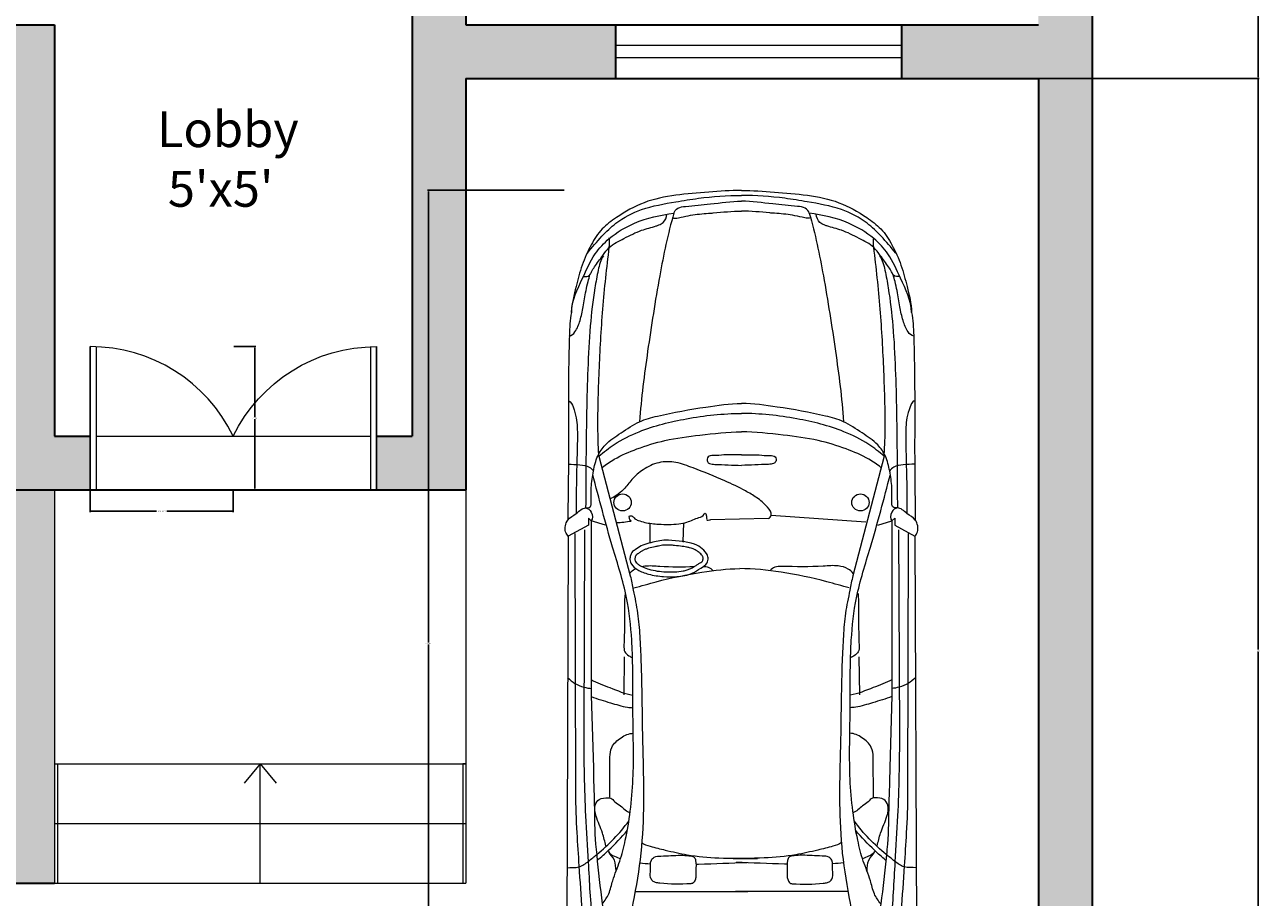
# Model space of a CAD drawing. Units: inches. Extents: x 1752 to 2227, y 6273 to 6884.
# Tile 3 of 6: x 2020 to 2227, y 6365 to 6511. Entities that reach past the tile are written whole.
import ezdxf

# ---------------------------------------------------------------- set-up
doc = ezdxf.new("R2010")
doc.units = ezdxf.units.IN
doc.header["$MEASUREMENT"] = 0
for name, color, linetype, lineweight in [('A-ANNO-DIMS', 2, 'Continuous', 18), ('A-AREA-IDEN', 7, 'Continuous', 18), ('A-DOOR', 3, 'Continuous', 20), ('A-EQPM-VEHI', 9, 'Continuous', 13), ('A-FLOR-STRS', 7, 'Continuous', 20), ('A-GLAZ', 4, 'Continuous', 18), ('A-WALL', 7, 'Continuous', 35)]:
    doc.layers.add(name, color=color, linetype=linetype, lineweight=lineweight)
doc.layers.add('A-WALL-PATT', color=32, linetype='Continuous', lineweight=13, true_color=0xcd6928)
doc.styles.get("Standard").update_dxf_attribs({"font": 'arial.ttf'})
doc.dimstyles.get("Standard").update_dxf_attribs({"dimtxt": 0.18, "dimasz": 0.18, "dimexe": 0.18, "dimexo": 0.0625, "dimgap": 0.09, "dimtad": 0, "dimtih": 1, "dimtoh": 1, "dimdec": 4, "dimzin": 0, "dimdsep": 46, "dimtxsty": 'Standard', "dimcen": 0.09, "dimadec": 0, "dimazin": 0, "dimtfac": 1, "dimtdec": 4, "dimtofl": 0, "dimtmove": 0, "dimatfit": 3, "dimfxl": 1, "dimtolj": 1, "dimtzin": 0, "dimarcsym": 0})

# ---------------------------------------------------------------- blocks, each defined once
blk = doc.blocks.new('A$C242571DA')
for p, q in [((1659.9, 1632), (1714.3, 1732.5)), ((1714.3, 1732.5), (3817.1, 1739.9)), ((1681.8, 1651.6), (2695.2, 1655.3)), ((1699.9, 1699.4), (2984.7, 1695.8)), ((1638.3, 1618.5), (1625.1, 1632)), ((1625.1, 1632), (1659.9, 1632)), ((1638.3, 1618.5), (2503.3, 1618.5)), ((1659.9, 1548.1), (1638.3, 1618.5)), ((2503.3, 1618.5), (2861.6, 1607.5)), ((1317.4, 1579.7), (1909.8, 1424.9)), ((1644, 1489.1), (1610.4, 1020.2)), ((3007.2, 1526.5), (2808.1, 1525.2)), ((2311.9, 1454.3), (2500.6, 1456.9)), ((3474.6, 1401.1), (3474.6, 843)), ((1626.1, 1006.5), (1632.8, 719.7)), ((3474.6, 345.6), (3474.6, 903.8)), ((1740.2, 584.9), (1649.3, 586.9)), ((1746.1, 420.6), (1649.3, 420.6)), ((1317.4, 167), (1909.8, 321.9)), ((2311.9, 292.5), (2500.6, 289.8)), ((1659.9, 198.7), (1638.3, 128.2)), ((3007.2, 220.3), (2808.1, 221.6)), ((1638.3, 128.2), (1625.1, 114.7)), ((1638.3, 128.2), (2503.3, 128.2)), ((2503.3, 128.2), (2861.6, 139.2)), ((1625.1, 114.7), (1659.9, 114.7)), ((1659.9, 114.7), (1714.3, 14.2)), ((1681.8, 95.1), (2695.2, 91.4)), ((1699.9, 47.3), (2984.7, 51)), ((1714.3, 14.2), (3817.1, 6.9))]:
    blk.add_line(p, q)
for centre in [(1546.4, 1462.5), (1546.4, 284.2)]:
    blk.add_ellipse(centre, major_axis=(0, 42.9), ratio=0.983266, start_param=4.712389, end_param=10.995574)
for points, knots in [([(0, 873.4), (0, 927.8), (15.6, 1088.6), (25.5, 1309.8), (120.7, 1476.4), (189.2, 1569), (273.5, 1623.1), (369.9, 1666.3), (483, 1694.7), (561.3, 1714.9), (604.6, 1715.7)], [0, 0, 0, 0, 0.16039, 0.479033, 0.632967, 0.722015, 0.817474, 0.927562, 1.03733, 1.167094, 1.167094, 1.167094, 1.167094]), ([(604.6, 1715.7), (545.5, 1714.5), (448.5, 1664.6), (320.8, 1610.6), (225.4, 1521.2), (147.3, 1390.5), (121.7, 1275.2), (113.6, 1208.7)], [0, 0, 0, 0, 0.1772572, 0.3124951, 0.4151678, 0.5597243, 0.7575412, 0.7575412, 0.7575412, 0.7575412]), ([(722.7, 1726.6), (720.8, 1714.9), (694.5, 1689.9), (643, 1671.8), (573.6, 1655.4), (508.5, 1647), (455.2, 1634.7), (428.7, 1627.3), (416.9, 1624.1)], [0, 0, 0, 0, 0.034703, 0.0959761, 0.1659336, 0.2471559, 0.2929944, 0.3295918, 0.3295918, 0.3295918, 0.3295918]), ([(604.6, 1715.7), (642.1, 1723.4), (788.5, 1729.2), (1039.3, 1732.2), (1344.5, 1729.9), (1542, 1733.1), (1633.8, 1733.7)], [0, 0, 0, 0, 0.114897, 0.437061, 0.754269, 1.029686, 1.029686, 1.029686, 1.029686]), ([(1043.6, 1729.2), (1048.6, 1717.9), (1080.9, 1704.2), (1138.6, 1687.6), (1237.7, 1685.6), (1394.7, 1691.3), (1521.7, 1692.4), (1601.5, 1692.7)], [0, 0, 0, 0, 0.0364992, 0.0923739, 0.1867837, 0.3273982, 0.5667068, 0.5667068, 0.5667068, 0.5667068]), ([(1356.8, 1732.2), (1357.1, 1712.8), (1360, 1678.8), (1363.9, 1630.5), (1383.3, 1613.5), (1391, 1607.2)], [0, 0, 0, 0, 1.462159, 2.651105, 3.386321, 3.386321, 3.386321, 3.386321]), ([(1714.3, 1732.5), (1707.7, 1737.6), (1683.3, 1753), (1628.7, 1741.2), (1605.6, 1691.5), (1561.7, 1652.4), (1594.1, 1610.3), (1627.9, 1608.3), (1638.3, 1618.5)], [0, 0, 0, 0, 0.024864, 0.0846267, 0.1362471, 0.1900683, 0.2245199, 0.2681841, 0.2681841, 0.2681841, 0.2681841]), ([(2414.7, 1735), (2424.9, 1723.3), (2447.2, 1698.8), (2461.2, 1657.6), (2468.1, 1629), (2468, 1616.1)], [1.808086, 1.808086, 1.808086, 1.808086, 2.918874, 4.131288, 5.10151, 5.10151, 5.10151, 5.10151]), ([(3356.5, 1739.4), (3354.9, 1719.2), (3360.8, 1678.2), (3324, 1631.5), (3255.4, 1544.3), (3187.1, 1476.2), (3125.2, 1432.2)], [0, 0, 0, 0, 0.0597371, 0.1139981, 0.1672498, 0.3938869, 0.3938869, 0.3938869, 0.3938869]), ([(426.8, 1656.7), (428.5, 1646.6), (426.9, 1625), (399.8, 1616.6), (368.1, 1593.9), (328, 1564.6), (271.6, 1523.9), (237, 1451.9), (196.2, 1376.7), (183.8, 1314.9), (170, 1279.6), (157.2, 1254.2), (133.3, 1244.4), (118.6, 1242.9)], [0, 0, 0, 0, 0.0304541, 0.0502818, 0.0786089, 0.1479133, 0.1986294, 0.2831705, 0.3780326, 0.4523267, 0.4667809, 0.4902599, 0.5347198, 0.5347198, 0.5347198, 0.5347198]), ([(2695.2, 1655.3), (2829.9, 1655.3), (3041.2, 1651.4), (3351.3, 1630.7), (3527.5, 1623.2), (3626.6, 1612)], [0, 0, 0, 0, 0.4042759, 0.6333827, 0.9326252, 0.9326252, 0.9326252, 0.9326252]), ([(2984.7, 1695.8), (3051, 1695.6), (3172.1, 1691.3), (3367.4, 1677.6), (3575.2, 1664.3), (3788.2, 1643.6), (3968, 1628.1), (4103.8, 1616.8), (4203.6, 1578.1), (4271.8, 1519.5), (4300.6, 1452.1), (4341.7, 1305.3), (4361.8, 1111.2), (4367.5, 936.8), (4367.5, 873.4)], [0, 0, 0, 0, 0.198873, 0.363323, 0.587433, 0.823543, 1.004622, 1.129816, 1.230113, 1.320655, 1.388577, 1.443334, 1.771447, 1.958652, 1.958652, 1.958652, 1.958652]), ([(310.7, 1637.3), (282.5, 1613.7), (230.1, 1569.9), (148.7, 1486.2), (84.8, 1361.3), (60, 1219), (32.6, 1054.3), (25.1, 944.9), (25.1, 873.4)], [0, 0, 0, 0, 0.1095129, 0.2035347, 0.3452507, 0.5161382, 0.6275464, 0.8383798, 0.8383798, 0.8383798, 0.8383798]), ([(323.7, 1557.5), (344.8, 1571.9), (400.4, 1585.1), (516, 1606.8), (680.3, 1625.8), (885.4, 1635.7), (1116.8, 1642.2), (1346.1, 1644.2), (1504.7, 1644.7), (1574, 1645.7)], [0, 0, 0, 0, 0.076148, 0.165903, 0.355672, 0.569871, 0.782325, 1.050047, 1.257936, 1.257936, 1.257936, 1.257936]), ([(1555.2, 1617.8), (1527.7, 1617.8), (1472.5, 1620.4), (1392.7, 1608.8), (1318.5, 1591), (1249.4, 1545.5), (1201.4, 1466.7), (1142.8, 1385.7), (1104.8, 1240.4), (1076, 1072.3), (1056.4, 932.4), (1056.4, 873.4)], [0, 0, 0, 0, 0.082256, 0.165174, 0.241383, 0.30939, 0.405348, 0.511507, 0.603349, 0.843635, 1.017671, 1.017671, 1.017671, 1.017671]), ([(3535.9, 1563.1), (3520.1, 1550.9), (3484.4, 1526.1), (3408.2, 1510.9), (3323.4, 1473.1), (3207.9, 1445), (3072.6, 1422.2), (2866.9, 1404.6), (2626.4, 1412.9), (2396.7, 1410.8), (2200.9, 1416.9), (2001.3, 1438.2), (1732.1, 1525.9), (1527.9, 1578.9), (1407.5, 1610.7)], [0, 0, 0, 0, 0.05975, 0.126928, 0.230034, 0.336675, 0.482225, 0.641324, 0.954906, 1.203173, 1.330375, 1.542773, 1.802261, 2.175545, 2.175545, 2.175545, 2.175545]), ([(1574, 1645.7), (1572.9, 1638), (1574.1, 1622), (1559.9, 1618.7), (1555.2, 1617.8)], [0, 0, 0, 0, 0.02274132, 0.03717479, 0.03717479, 0.03717479, 0.03717479]), ([(2424, 1618.7), (2441.5, 1589.9), (2464.2, 1518.9), (2495.4, 1450.9), (2501.6, 1411.3)], [0, 0, 0, 0, 0.1000351, 0.2184418, 0.2184418, 0.2184418, 0.2184418]), ([(2507.7, 1618.4), (2521, 1587.7), (2536.6, 1527.1), (2559.6, 1458.5), (2563.3, 1420.6), (2563.8, 1411.4)], [0, 0, 0, 0, 2.528586, 4.711885, 5.408215, 5.408215, 5.408215, 5.408215]), ([(2861.6, 1607.5), (2921.1, 1607.3), (3047.2, 1600.8), (3191.4, 1602), (3356.6, 1584.1), (3498.3, 1570.6), (3623.2, 1549.4), (3664.1, 1533.3)], [0, 0, 0, 0, 0.1783018, 0.3787173, 0.431954, 0.6762374, 0.8077184, 0.8077184, 0.8077184, 0.8077184]), ([(3248.1, 1545.2), (3226.9, 1550.4), (3176.1, 1562.1), (3113.7, 1592.9), (3052.6, 1605.3), (3010.4, 1578.8), (3010.3, 1545.3), (3010.3, 1515.9), (3033.7, 1500.1), (3052.6, 1465.2), (3078.9, 1443.5), (3084, 1424.4)], [0, 0, 0, 0, 0.0655106, 0.1550445, 0.2094604, 0.2438604, 0.287164, 0.3001388, 0.3275984, 0.3616951, 0.4200969, 0.4200969, 0.4200969, 0.4200969]), ([(1317.4, 1579.7), (1227.8, 1586.1), (1036, 1584.8), (741.2, 1572.5), (486.1, 1553.3), (333.3, 1534.3), (283.3, 1528.5)], [0, 0, 0, 0, 0.269375, 0.574535, 0.885339, 1.036319, 1.036319, 1.036319, 1.036319]), ([(1317.4, 1579.7), (1296.6, 1555.5), (1247.9, 1494.4), (1177.6, 1350.5), (1124.2, 1137.4), (1105.5, 964.9), (1105.5, 873.4)], [0, 0, 0, 0, 0.0947759, 0.2311242, 0.4700259, 0.7400315, 0.7400315, 0.7400315, 0.7400315]), ([(1372.8, 1563.1), (1357.2, 1545), (1321.6, 1490.1), (1277, 1385.7), (1232.8, 1244.2), (1211.1, 1069.4), (1196.8, 942.4), (1196.8, 873.4)], [0, 0, 0, 0, 0.0708922, 0.1925846, 0.3348457, 0.5072814, 0.7109928, 0.7109928, 0.7109928, 0.7109928]), ([(3319, 1587.1), (3303.3, 1568.1), (3256.9, 1516.7), (3206.7, 1467.3), (3171.4, 1439.5)], [0, 0, 0, 0, 1.868162, 5.271297, 5.271297, 5.271297, 5.271297]), ([(3275.5, 1532.8), (3287.5, 1528.3), (3299.8, 1504.9), (3308.4, 1482.5), (3311.7, 1472.6)], [0, 0, 0, 0, 0.983949, 1.771691, 1.771691, 1.771691, 1.771691]), ([(3372.2, 1495.3), (3354.4, 1496.8), (3316, 1494.7), (3291.6, 1525.8), (3275.5, 1532.8)], [0, 0, 0, 0, 0.0535488, 0.1060573, 0.1060573, 0.1060573, 0.1060573]), ([(2808.1, 1525.2), (2791.9, 1525.1), (2751.9, 1519.7), (2710.6, 1472.6), (2690, 1431.1), (2690.5, 1409.6)], [0, 0, 0, 0, 0.0486628, 0.1144515, 0.1777721, 0.1777721, 0.1777721, 0.1777721]), ([(1898.5, 1426.2), (1889, 1420.6), (1871, 1397.2), (1856.4, 1345.2), (1867.7, 1233.5), (1864.3, 1132.3), (1863, 1038.5), (1876.9, 1022.3), (1884.5, 1015.7)], [0, 0, 0, 0, 0.842998, 2.122875, 3.997599, 9.174838, 10.012722, 10.751336, 10.751336, 10.751336, 10.751336]), ([(1969.6, 1407.3), (1960.5, 1369.8), (1927, 1259.1), (1890.9, 1078.4), (1874.3, 933), (1874.3, 864.4)], [0, 0, 0, 0, 0.1139079, 0.3411539, 0.543502, 0.543502, 0.543502, 0.543502]), ([(1909.8, 1424.9), (1933.5, 1418.7), (1995.6, 1407.6), (2094.4, 1385.8), (2211.8, 1377.1), (2419, 1366.9), (2704.7, 1366.5), (3032.7, 1354.2), (3316.2, 1371), (3558.7, 1415.9), (3789.1, 1461.7), (4028.9, 1452.9), (4196.2, 1455.2), (4292.7, 1447.9), (4300.7, 1447.5)], [0, 0, 0, 0, 0.073325, 0.188896, 0.303039, 0.425821, 0.811242, 1.159737, 1.41058, 1.660623, 1.899627, 2.11145, 2.377727, 2.401703, 2.401703, 2.401703, 2.401703]), ([(1997.2, 1450.5), (2039.7, 1454.5), (2126.7, 1451.9), (2219.8, 1454.5), (2287.1, 1456.9), (2305.7, 1434.4), (2313.2, 1419.9), (2315.8, 1413.5)], [0, 0, 0, 0, 3.267856, 6.568708, 7.399663, 8.099385, 8.621705, 8.621705, 8.621705, 8.621705]), ([(113.6, 1208.7), (215.2, 1238.6), (443.2, 1284.9), (788, 1338.7), (1029.5, 1370.7), (1146.4, 1378.6)], [0, 0, 0, 0, 0.317374, 0.69576, 1.04714, 1.04714, 1.04714, 1.04714]), ([(3231.5, 1368.3), (3240.8, 1356.2), (3253.1, 1315.7), (3271.9, 1240.7), (3297.9, 1127.9), (3310.5, 974.6), (3311.2, 858.3), (3311.6, 794.4)], [0, 0, 0, 0, 0.0451009, 0.1211996, 0.2308505, 0.385263, 0.5739042, 0.5739042, 0.5739042, 0.5739042]), ([(3294.8, 1174.5), (3294.8, 1207.4), (3299.6, 1249.5), (3298.3, 1303.9), (3326.3, 1329), (3363.9, 1320.7), (3399.3, 1329.3), (3422.1, 1315.7), (3430.7, 1297.9), (3438.7, 1234.2), (3439.6, 1174.4), (3434.7, 1112.2), (3418.9, 1102), (3395.9, 1098.6), (3362.6, 1100.9), (3331.1, 1096.6), (3298.8, 1107.6), (3297.3, 1140.3), (3294.8, 1160.9), (3294.8, 1174.5)], [0, 0, 0, 0, 0.0969044, 0.1295913, 0.1506192, 0.1985921, 0.2360698, 0.2557908, 0.2719711, 0.2929882, 0.44406, 0.4519132, 0.4720918, 0.4918599, 0.5228758, 0.5707096, 0.5892096, 0.6145759, 0.654681, 0.654681, 0.654681, 0.654681]), ([(113.6, 1208.7), (103.3, 1207), (83.6, 1187.6), (76.5, 1122.2), (68.2, 1017.3), (53.4, 925), (53.4, 873.4)], [0, 0, 0, 0, 0.0314754, 0.0702057, 0.1915753, 0.3439346, 0.3439346, 0.3439346, 0.3439346]), ([(135.5, 1213.1), (139.1, 1211.8), (138.4, 1193.3), (132.6, 1168.3), (118.8, 1111.9), (115.6, 1058.9), (109, 974.6), (102.4, 920.1), (102.4, 873.4)], [0, 0, 0, 0, 0.0114788, 0.0403472, 0.0875838, 0.1755608, 0.1991501, 0.3369659, 0.3369659, 0.3369659, 0.3369659]), ([(1311.3, 873.4), (1311.2, 902.4), (1309.2, 950.9), (1315, 1002.2), (1314.2, 1039.4), (1332.1, 1044.9), (1345.7, 1044.2), (1356.8, 1028.5), (1359.2, 970.2), (1361.5, 917.6), (1362.9, 873.4)], [0, 0, 0, 0, 0.0857277, 0.1381048, 0.1641986, 0.1769751, 0.1890325, 0.2028129, 0.2286049, 0.3592554, 0.3592554, 0.3592554, 0.3592554]), ([(3339.2, 1099), (3339.1, 1094.8), (3336.4, 1010.6), (3333.2, 926.3), (3330, 846.2)], [11.235438, 11.235438, 11.235438, 11.235438, 11.552536, 17.586883, 17.586883, 17.586883, 17.586883]), ([(1626.1, 1006.5), (1623.5, 1013), (1603.1, 1029.4), (1559.1, 995), (1523, 951.9), (1480.3, 878.3), (1430.5, 774.3), (1385.5, 658.5), (1343.7, 551.3), (1343, 461.7), (1380.3, 386.9), (1428.2, 329.9), (1480.1, 294.6), (1509.8, 257.4), (1524.8, 232.6), (1528, 222.1)], [0, 0, 0, 0, 0.527288, 1.647451, 3.487558, 5.099073, 7.968657, 12.238313, 14.475187, 16.613757, 18.744202, 20.639343, 22.223389, 23.452731, 24.286529, 24.286529, 24.286529, 24.286529]), ([(3231.5, 378.5), (3240.8, 390.5), (3253.1, 431), (3271.9, 506.1), (3297.9, 618.9), (3310.5, 772.1), (3311.2, 888.4), (3311.6, 952.4)], [0, 0, 0, 0, 0.0451009, 0.1211996, 0.2308505, 0.385263, 0.5739042, 0.5739042, 0.5739042, 0.5739042]), ([(0, 873.4), (0, 819), (15.6, 658.1), (25.5, 437), (120.7, 270.3), (189.2, 177.8), (273.5, 123.7), (369.9, 80.4), (483, 52), (561.3, 31.9), (604.6, 31)], [0, 0, 0, 0, 0.16039, 0.479033, 0.632967, 0.722015, 0.817474, 0.927562, 1.03733, 1.167094, 1.167094, 1.167094, 1.167094]), ([(310.7, 109.5), (282.5, 133.1), (230.1, 176.9), (148.7, 260.5), (84.8, 385.5), (60, 527.8), (32.6, 692.4), (25.1, 801.9), (25.1, 873.4)], [0, 0, 0, 0, 0.1095129, 0.2035347, 0.3452507, 0.5161382, 0.6275464, 0.8383798, 0.8383798, 0.8383798, 0.8383798]), ([(113.6, 538.1), (103.3, 539.8), (83.6, 559.2), (76.5, 624.5), (68.2, 729.4), (53.4, 821.7), (53.4, 873.4)], [0, 0, 0, 0, 0.0314754, 0.0702057, 0.1915753, 0.3439346, 0.3439346, 0.3439346, 0.3439346]), ([(135.5, 533.6), (139.1, 534.9), (138.4, 553.4), (132.6, 578.4), (118.8, 634.9), (115.6, 687.8), (109, 772.2), (102.4, 826.7), (102.4, 873.4)], [0, 0, 0, 0, 0.0114788, 0.0403472, 0.0875838, 0.1755608, 0.1991501, 0.3369659, 0.3369659, 0.3369659, 0.3369659]), ([(1555.2, 129), (1527.7, 129), (1472.5, 126.3), (1392.7, 138), (1318.5, 155.7), (1249.4, 201.3), (1201.4, 280.1), (1142.8, 361.1), (1104.8, 506.4), (1076, 674.5), (1056.4, 814.4), (1056.4, 873.4)], [0, 0, 0, 0, 0.082256, 0.165174, 0.241383, 0.30939, 0.405348, 0.511507, 0.603349, 0.843635, 1.017671, 1.017671, 1.017671, 1.017671]), ([(1317.4, 167), (1296.6, 191.2), (1247.9, 252.4), (1177.6, 396.3), (1124.2, 609.4), (1105.5, 781.8), (1105.5, 873.4)], [0, 0, 0, 0, 0.0947759, 0.2311242, 0.4700259, 0.7400315, 0.7400315, 0.7400315, 0.7400315]), ([(1372.8, 183.6), (1357.2, 201.8), (1321.6, 256.7), (1277, 361), (1232.8, 502.6), (1211.1, 677.3), (1196.8, 804.3), (1196.8, 873.4)], [0, 0, 0, 0, 0.0708922, 0.1925846, 0.3348457, 0.5072814, 0.7109928, 0.7109928, 0.7109928, 0.7109928]), ([(1311.3, 873.4), (1311.2, 844.3), (1309.2, 795.8), (1315, 744.6), (1314.2, 707.4), (1332.1, 701.9), (1345.7, 702.6), (1356.8, 718.2), (1359.2, 776.6), (1361.5, 829.1), (1362.9, 873.4)], [0, 0, 0, 0, 0.0857277, 0.1381048, 0.1641986, 0.1769751, 0.1890325, 0.2028129, 0.2286049, 0.3592554, 0.3592554, 0.3592554, 0.3592554]), ([(1969.6, 339.5), (1960.5, 377), (1926.9, 487.6), (1892.9, 662.7), (1874.3, 801.8), (1874.3, 864.4)], [0, 0, 0, 0, 0.1139079, 0.3411539, 0.5260188, 0.5260188, 0.5260188, 0.5260188]), ([(2984.7, 51), (3051, 51.1), (3172.1, 55.5), (3367.4, 69.2), (3575.2, 82.5), (3788.2, 103.1), (3968, 118.7), (4103.8, 130), (4203.6, 168.6), (4271.8, 227.3), (4300.6, 294.7), (4341.7, 441.5), (4361.8, 635.5), (4367.5, 809.9), (4367.5, 873.4)], [0, 0, 0, 0, 0.198873, 0.363323, 0.587433, 0.823543, 1.004622, 1.129816, 1.230113, 1.320655, 1.388577, 1.443334, 1.771447, 1.958652, 1.958652, 1.958652, 1.958652]), ([(3339.2, 647.8), (3339.1, 652), (3336.4, 736.2), (3333.2, 820.5), (3330, 900.6)], [11.235438, 11.235438, 11.235438, 11.235438, 11.552536, 17.586883, 17.586883, 17.586883, 17.586883]), ([(1639.2, 326.1), (1635.3, 323.6), (1629, 318.4), (1613.1, 314.9), (1612, 324.2), (1613.2, 330.4), (1619, 337.5), (1629, 345.7), (1637.9, 366.1), (1649, 404.8), (1656.3, 472.9), (1656.2, 543.1), (1644.6, 610.9), (1623, 651.2), (1615, 684.3), (1598.5, 691.2), (1604, 696.6), (1610.3, 699.7), (1618.8, 698.9), (1625.9, 701.3), (1638.1, 698.6), (1633, 713.4), (1632.8, 719.7)], [0, 0, 0, 0, 0.0138597, 0.0278304, 0.0329137, 0.0379971, 0.0465756, 0.0592704, 0.0762214, 0.1105991, 0.1789801, 0.2766959, 0.3173629, 0.3800771, 0.4110544, 0.4160421, 0.4210284, 0.4277212, 0.4387433, 0.4448131, 0.4508005, 0.4694463, 0.4694463, 0.4694463, 0.4694463]), ([(1740.2, 584.9), (1737.8, 571.7), (1749.5, 644.3), (1766.4, 664.5), (1792.2, 700.2), (1821.5, 709.7), (1853.1, 703.9), (1874, 668.4), (1904.5, 622.6), (1915.6, 557.2), (1915.1, 484.2), (1905.7, 417.6), (1884.9, 362.8), (1859.3, 329.1), (1831.3, 318.1), (1810.8, 322.7), (1792.2, 329.3), (1777.9, 350.3), (1753, 385.9), (1737.9, 465.8), (1728.8, 497.3), (1742.4, 597.6), (1740.2, 584.9)], [0, 0, 0, 0, 0.03969, 0.089634, 0.13125, 0.1542862, 0.1797268, 0.2207266, 0.2680991, 0.3447665, 0.4095645, 0.4843001, 0.541515, 0.5817687, 0.6060665, 0.6262474, 0.6436722, 0.6634686, 0.6988791, 0.7758465, 0.8696394, 0.907731, 0.907731, 0.907731, 0.907731]), ([(1764.9, 587), (1765.6, 590.8), (1766.4, 595.5), (1768.5, 605.7), (1769.7, 611.3), (1773.4, 626.6), (1775.6, 633), (1779.7, 642.1), (1781.6, 644.9), (1785.7, 650.6), (1787.1, 652.5), (1793, 660.3), (1797.4, 666.2), (1804.2, 673.7), (1806.8, 676.1), (1811.1, 679.4), (1812.9, 680.5), (1816.8, 682.1), (1818.8, 682.7), (1824.4, 683.5), (1828.3, 683.2), (1832.5, 682), (1833.6, 681.5), (1836, 680.2), (1837.9, 678.7), (1842.4, 673.7), (1844.9, 670.1), (1850.3, 661.7), (1853.4, 656.6), (1859.3, 647.3), (1862.1, 642.8), (1868.3, 632.6), (1871.4, 626.9), (1876.7, 615.7), (1878.9, 609.8), (1882.8, 597.4), (1884.4, 590.8), (1888.3, 570.5), (1889.7, 556.1), (1891.2, 527.4), (1891.1, 513.1), (1888.9, 470), (1885.1, 441.2), (1874.3, 404), (1870.6, 393.8), (1863.5, 378.7), (1860.6, 373.4), (1854.4, 363.6), (1851.2, 359.2), (1845, 352.6), (1842, 350.2), (1835.8, 346.4), (1832.6, 345.3), (1828.8, 344.6), (1827.9, 344.6), (1824.6, 344.9), (1822.6, 345.2), (1817.8, 346.4), (1814.9, 347.3), (1810.9, 348.7), (1809.4, 349.4), (1808.3, 350.1), (1808.1, 350.2), (1807.3, 351), (1806.7, 351.6), (1804.7, 354), (1803.1, 356.2), (1799.6, 361.3), (1798, 363.7), (1794.9, 368.2), (1793.4, 370.4), (1789.2, 376.9), (1786.7, 381), (1782.4, 389.3), (1780.5, 393.6), (1776.9, 403), (1775.2, 408), (1770.7, 423.5), (1768.3, 434.2), (1764.9, 450.5), (1763.6, 456.4), (1761.4, 466.8), (1760.4, 471.4), (1758.1, 484.4), (1757.3, 492.6), (1757.5, 510.7), (1757.8, 516.5), (1758.6, 528.4), (1759.1, 534.3), (1761.1, 553.9), (1763.1, 570.6), (1764.4, 581.5), (1764.6, 583), (1764.7, 585), (1764.8, 585.5), (1764.8, 586.5), (1764.8, 586.7), (1764.9, 587)], [0.497033, 0.497033, 0.497033, 0.497033, 0.723444, 0.723444, 0.974636, 0.974636, 1.50964, 1.50964, 2.044645, 2.044645, 2.271061, 2.271061, 2.862376, 2.862376, 3.217654, 3.217654, 3.537253, 3.537253, 3.856852, 3.856852, 4.368613, 4.368613, 4.584627, 4.584627, 4.99269, 4.99269, 5.400753, 5.400753, 5.808816, 5.808816, 6.216879, 6.216879, 6.778716, 6.778716, 7.350371, 7.350371, 7.922025, 7.922025, 9.065335, 9.065335, 10.208644, 10.208644, 12.495263, 12.495263, 13.409896, 13.409896, 13.929088, 13.929088, 14.44828, 14.44828, 14.909885, 14.909885, 15.371489, 15.371489, 15.62524, 15.62524, 15.87899, 15.87899, 16.120875, 16.120875, 16.36276, 16.36276, 16.51635, 16.51635, 16.669941, 16.669941, 16.921521, 16.921521, 17.136676, 17.136676, 17.351831, 17.351831, 17.782142, 17.782142, 18.204974, 18.204974, 18.627807, 18.627807, 19.473473, 19.473473, 19.978923, 19.978923, 20.484372, 20.484372, 21.475119, 21.475119, 21.859144, 21.859144, 22.162884, 22.162884, 22.770362, 22.770362, 22.900493, 22.900493, 22.951221, 22.951221, 22.964298, 22.964298, 22.964298, 22.964298]), ([(1863.4, 685.6), (1863.6, 693.5), (1865.3, 711), (1876.9, 724.5), (1884.5, 731)], [9.436432, 9.436432, 9.436432, 9.436432, 10.012722, 10.751336, 10.751336, 10.751336, 10.751336]), ([(1863.7, 379.4), (1862.6, 384.2), (1857.6, 413.7), (1866.5, 501.6), (1865.2, 581.4), (1864.1, 639.5)], [1.749253, 1.749253, 1.749253, 1.749253, 2.122875, 3.997599, 8.307432, 8.307432, 8.307432, 8.307432]), ([(3294.8, 572.3), (3294.8, 539.4), (3299.6, 497.2), (3298.3, 442.9), (3326.3, 417.8), (3363.9, 426), (3399.3, 417.5), (3422.1, 431), (3430.7, 448.9), (3438.7, 512.5), (3439.6, 572.4), (3434.7, 634.6), (3418.9, 644.7), (3395.9, 648.2), (3362.6, 645.9), (3331.1, 650.1), (3298.8, 639.2), (3297.3, 606.5), (3294.8, 585.9), (3294.8, 572.3)], [0, 0, 0, 0, 0.0969044, 0.1295913, 0.1506192, 0.1985921, 0.2360698, 0.2557908, 0.2719711, 0.2929882, 0.44406, 0.4519132, 0.4720918, 0.4918599, 0.5228758, 0.5707096, 0.5892096, 0.6145759, 0.654681, 0.654681, 0.654681, 0.654681]), ([(604.6, 31), (545.5, 32.3), (448.5, 82.2), (320.8, 136.1), (225.4, 225.5), (147.3, 356.2), (121.7, 471.5), (113.6, 538.1)], [0, 0, 0, 0, 0.1772572, 0.3124951, 0.4151678, 0.5597243, 0.7575412, 0.7575412, 0.7575412, 0.7575412]), ([(113.6, 538.1), (215.2, 508.2), (443.2, 461.9), (788, 408.1), (1029.5, 376), (1146.4, 368.2)], [0, 0, 0, 0, 0.317374, 0.69576, 1.04714, 1.04714, 1.04714, 1.04714]), ([(426.8, 90), (428.5, 100.2), (426.9, 121.8), (399.8, 130.1), (368.1, 152.8), (328, 182.2), (271.6, 222.8), (237, 294.9), (196.2, 370.1), (183.8, 431.9), (170, 467.2), (157.2, 492.6), (133.3, 502.4), (118.6, 503.9)], [0, 0, 0, 0, 0.0304541, 0.0502818, 0.0786089, 0.1479133, 0.1986294, 0.2831705, 0.3780326, 0.4523267, 0.4667809, 0.4902599, 0.5347198, 0.5347198, 0.5347198, 0.5347198]), ([(1909.8, 321.9), (1933.5, 328.1), (1995.6, 339.2), (2094.4, 361), (2211.8, 369.6), (2419, 379.8), (2704.7, 380.3), (3032.7, 392.6), (3316.2, 375.8), (3558.7, 330.9), (3789.1, 285.1), (4028.9, 293.9), (4196.2, 291.5), (4292.7, 298.8), (4300.7, 299.2)], [0, 0, 0, 0, 0.073325, 0.188896, 0.303039, 0.425821, 0.811242, 1.159737, 1.41058, 1.660623, 1.899627, 2.11145, 2.377727, 2.401703, 2.401703, 2.401703, 2.401703]), ([(3535.9, 183.7), (3520.1, 195.9), (3484.4, 220.6), (3408.2, 235.8), (3323.4, 273.7), (3207.9, 301.8), (3072.6, 324.6), (2866.9, 342.1), (2626.4, 333.8), (2396.7, 335.9), (2200.9, 329.9), (2001.3, 308.6), (1732.1, 220.8), (1527.9, 167.8), (1407.5, 136)], [0, 0, 0, 0, 0.05975, 0.126928, 0.230034, 0.336675, 0.482225, 0.641324, 0.954906, 1.203173, 1.330375, 1.542773, 1.802261, 2.175545, 2.175545, 2.175545, 2.175545]), ([(1898.5, 320.6), (1889, 326.2), (1880.8, 336.8), (1874.8, 348.3), (1874, 349.7)], [0, 0, 0, 0, 0.8429982, 0.9626806, 0.9626806, 0.9626806, 0.9626806]), ([(1997.2, 296.3), (2039.7, 292.2), (2126.7, 294.9), (2219.8, 292.3), (2287.1, 289.9), (2305.7, 312.3), (2313.2, 326.9), (2315.8, 333.2)], [0, 0, 0, 0, 3.267856, 6.568708, 7.399663, 8.099385, 8.621705, 8.621705, 8.621705, 8.621705]), ([(2424, 128), (2441.5, 156.9), (2464.2, 227.8), (2495.4, 295.8), (2501.6, 335.5)], [0, 0, 0, 0, 0.1000351, 0.2184418, 0.2184418, 0.2184418, 0.2184418]), ([(2507.7, 128.3), (2521, 159.1), (2536.6, 219.7), (2559.6, 288.3), (2563.3, 326.1), (2563.8, 335.3)], [0, 0, 0, 0, 2.528586, 4.711885, 5.408215, 5.408215, 5.408215, 5.408215]), ([(2808.1, 221.6), (2791.9, 221.6), (2751.9, 227.1), (2710.6, 274.2), (2690, 315.7), (2690.5, 337.1)], [0, 0, 0, 0, 0.0486628, 0.1144515, 0.1777721, 0.1777721, 0.1777721, 0.1777721]), ([(3248.1, 201.6), (3226.9, 196.3), (3176.1, 184.7), (3113.7, 153.8), (3052.6, 141.4), (3010.4, 168), (3010.3, 201.5), (3010.3, 230.9), (3033.7, 246.6), (3052.6, 281.6), (3078.9, 303.2), (3084, 322.4)], [0, 0, 0, 0, 0.0655106, 0.1550445, 0.2094604, 0.2438604, 0.287164, 0.3001388, 0.3275984, 0.3616951, 0.4200969, 0.4200969, 0.4200969, 0.4200969]), ([(3356.5, 7.4), (3354.9, 27.5), (3360.8, 68.5), (3324, 115.2), (3255.4, 202.5), (3187.1, 270.5), (3125.2, 314.6)], [0, 0, 0, 0, 0.0597371, 0.1139981, 0.1672498, 0.3938869, 0.3938869, 0.3938869, 0.3938869]), ([(3319, 159.7), (3303.3, 178.6), (3256.9, 230), (3206.7, 279.5), (3171.4, 307.2)], [0, 0, 0, 0, 1.868162, 5.271297, 5.271297, 5.271297, 5.271297]), ([(3275.5, 214), (3287.5, 218.5), (3299.8, 241.9), (3308.4, 264.3), (3311.7, 274.2)], [0, 0, 0, 0, 0.983949, 1.771691, 1.771691, 1.771691, 1.771691]), ([(3372.2, 251.5), (3354.4, 249.9), (3316, 252), (3291.6, 220.9), (3275.5, 214)], [0, 0, 0, 0, 0.0535488, 0.1060573, 0.1060573, 0.1060573, 0.1060573]), ([(1317.4, 167), (1227.8, 160.7), (1036, 161.9), (741.2, 174.2), (486.1, 193.4), (333.3, 212.5), (283.3, 218.3)], [0, 0, 0, 0, 0.269375, 0.574535, 0.885339, 1.036319, 1.036319, 1.036319, 1.036319]), ([(323.7, 189.2), (344.8, 174.9), (400.4, 161.7), (516, 139.9), (680.3, 121), (885.4, 111), (1116.8, 104.5), (1346.1, 102.5), (1504.7, 102), (1574, 101.1)], [0, 0, 0, 0, 0.076148, 0.165903, 0.355672, 0.569871, 0.782325, 1.050047, 1.257936, 1.257936, 1.257936, 1.257936]), ([(2861.6, 139.2), (2921.1, 139.4), (3047.2, 146), (3191.4, 144.8), (3356.6, 162.6), (3498.3, 176.1), (3623.2, 197.4), (3664.1, 213.5)], [0, 0, 0, 0, 0.1783018, 0.3787173, 0.431954, 0.6762374, 0.8077184, 0.8077184, 0.8077184, 0.8077184]), ([(722.7, 20.2), (720.8, 31.8), (694.5, 56.8), (643, 75), (573.6, 91.4), (508.5, 99.8), (455.2, 112.1), (428.7, 119.5), (416.9, 122.6)], [0, 0, 0, 0, 0.034703, 0.0959761, 0.1659336, 0.2471559, 0.2929944, 0.3295918, 0.3295918, 0.3295918, 0.3295918]), ([(1356.8, 14.5), (1357.1, 33.9), (1360, 68), (1363.9, 116.3), (1383.3, 133.2), (1391, 139.5)], [0, 0, 0, 0, 1.462159, 2.651105, 3.386321, 3.386321, 3.386321, 3.386321]), ([(1574, 101.1), (1572.9, 108.7), (1574.1, 124.8), (1559.9, 128), (1555.2, 129)], [0, 0, 0, 0, 0.02274132, 0.03717479, 0.03717479, 0.03717479, 0.03717479]), ([(1714.3, 14.2), (1707.7, 9.2), (1683.3, -6.3), (1628.7, 5.5), (1605.6, 55.3), (1561.7, 94.4), (1594.1, 136.5), (1627.9, 138.5), (1638.3, 128.2)], [0, 0, 0, 0, 0.024864, 0.0846267, 0.1362471, 0.1900683, 0.2245199, 0.2681841, 0.2681841, 0.2681841, 0.2681841]), ([(2414.7, 11.8), (2424.9, 23.5), (2447.2, 48), (2461.2, 89.1), (2468.1, 117.8), (2468, 130.7)], [1.808086, 1.808086, 1.808086, 1.808086, 2.918874, 4.131288, 5.10151, 5.10151, 5.10151, 5.10151]), ([(2695.2, 91.4), (2829.9, 91.5), (3041.2, 95.4), (3351.3, 116.1), (3527.5, 123.5), (3626.6, 134.7)], [0, 0, 0, 0, 0.4042759, 0.6333827, 0.9326252, 0.9326252, 0.9326252, 0.9326252]), ([(604.6, 31), (642.1, 23.4), (788.5, 17.5), (1039.3, 14.6), (1344.5, 16.8), (1542, 13.6), (1633.8, 13.1)], [0, 0, 0, 0, 0.114897, 0.437061, 0.754269, 1.029686, 1.029686, 1.029686, 1.029686]), ([(1043.6, 17.6), (1048.6, 28.9), (1080.9, 42.6), (1138.6, 59.2), (1237.7, 61.2), (1394.7, 55.4), (1521.7, 54.3), (1601.5, 54.1)], [0, 0, 0, 0, 0.0364992, 0.0923739, 0.1867837, 0.3273982, 0.5667068, 0.5667068, 0.5667068, 0.5667068])]:
    blk.add_open_spline(points, degree=3, knots=knots)
for points in [[(283.3, 1528.5), (267.8, 1524.6), (251.4, 1527.5), (235.4, 1528.5)], [(3331.9, 1378.1), (3334.2, 1360.4), (3335.9, 1342.5), (3337.3, 1324.5)], [(3331.9, 368.6), (3334.2, 386.4), (3335.9, 404.3), (3337.3, 422.2)], [(1646.2, 253.1), (1647.8, 277.5), (1640, 301.6), (1639.2, 326.1)], [(283.3, 218.3), (267.8, 222.1), (251.4, 219.2), (235.4, 218.3)]]:
    blk.add_open_spline(points, degree=3)
blk = doc.blocks.new('DOOR-PAIRED-24IN-LEAF')
for p, q in [((0, 0), (0, 24)), ((1, 24), (1, 0))]:
    blk.add_line(p, q)
blk.add_arc((0, -2.7), 26.7, 25.9892, 90)
blk = doc.blocks.new('WINDOW-48IN')
for p, q in [((48, 9), (0, 9)), ((48, 5.5), (0, 5.5)), ((0, 3.5), (48, 3.5)), ((0, 0), (48, 0))]:
    blk.add_line(p, q)
blk = doc.blocks.new('*D32')
at = {"layer": 'A-ANNO-DIMS', "color": 0, "lineweight": -2, "transparency": 16777216}
for p, q in [((2030.65, 6432.85), (2030.65, 6429.13)), ((2054.65, 6432.85), (2054.65, 6429.13)), ((2030.83, 6429.31), (2041.77, 6429.31)), ((2054.47, 6429.31), (2043.52, 6429.31))]:
    blk.add_line(p, q, dxfattribs=at)
at = {"layer": 'A-ANNO-DIMS', "color": 0, "transparency": 16777216}
for points in [[(2030.83, 6429.34), (2030.83, 6429.28), (2030.65, 6429.31)], [(2054.47, 6429.34), (2054.47, 6429.28), (2054.65, 6429.31)]]:
    blk.add_solid(points, dxfattribs=at)
at = {"layer": 'Defpoints', "color": 0, "transparency": 16777216}
for p in [(2030.65, 6432.91), (2054.65, 6432.91), (2054.65, 6429.31)]:
    blk.add_point(p, dxfattribs=at)
at = {"layer": 'A-ANNO-DIMS', "color": 0, "transparency": 16777216, "insert": (2042.65, 6429.31), "char_height": 0.18, "attachment_point": 5}
blk.add_mtext('\\A1;LEAF 24 TYP.', dxfattribs=at)
blk = doc.blocks.new('*D33')
at = {"layer": 'A-ANNO-DIMS', "color": 0, "lineweight": -2, "transparency": 16777216}
for p, q in [((2054.71, 6456.91), (2058.43, 6456.91)), ((2058.25, 6456.73), (2058.25, 6445.09)), ((2058.25, 6433.09), (2058.25, 6444.73)), ((2054.71, 6432.91), (2058.43, 6432.91))]:
    blk.add_line(p, q, dxfattribs=at)
at = {"layer": 'A-ANNO-DIMS', "color": 0, "transparency": 16777216}
for points in [[(2058.22, 6456.73), (2058.28, 6456.73), (2058.25, 6456.91)], [(2058.22, 6433.09), (2058.28, 6433.09), (2058.25, 6432.91)]]:
    blk.add_solid(points, dxfattribs=at)
at = {"layer": 'Defpoints', "color": 0, "transparency": 16777216}
for p in [(2054.65, 6456.91), (2058.25, 6456.91), (2054.65, 6432.91)]:
    blk.add_point(p, dxfattribs=at)
at = {"layer": 'A-ANNO-DIMS', "color": 0, "transparency": 16777216, "insert": (2058.25, 6444.91), "char_height": 0.18, "attachment_point": 5}
blk.add_mtext('\\A1;24 TYP.', dxfattribs=at)
blk = doc.blocks.new('*D38')
at = {"layer": 'A-ANNO-DIMS', "color": 0, "lineweight": -2, "transparency": 16777216}
for p, q in [((2110.11, 6483.13), (2087.19, 6483.13)), ((2087.37, 6482.95), (2087.37, 6407.29)), ((2087.37, 6331.28), (2087.37, 6406.93)), ((2110.11, 6331.1), (2087.19, 6331.1))]:
    blk.add_line(p, q, dxfattribs=at)
at = {"layer": 'A-ANNO-DIMS', "color": 0, "transparency": 16777216}
for points in [[(2087.34, 6482.95), (2087.4, 6482.95), (2087.37, 6483.13)], [(2087.34, 6331.28), (2087.4, 6331.28), (2087.37, 6331.1)]]:
    blk.add_solid(points, dxfattribs=at)
at = {"layer": 'Defpoints', "color": 0, "transparency": 16777216}
for p in [(2110.17, 6483.13), (2087.37, 6331.1), (2110.17, 6331.1)]:
    blk.add_point(p, dxfattribs=at)
at = {"layer": 'A-ANNO-DIMS', "color": 0, "transparency": 16777216, "insert": (2087.37, 6407.11), "char_height": 0.18, "attachment_point": 5}
blk.add_mtext('\\A1;CAR 152', dxfattribs=at)
blk = doc.blocks.new('*D42')
at = {"layer": 'A-ANNO-DIMS', "color": 0, "lineweight": -2, "transparency": 16777216}
for p, q in [((2189.71, 6501.91), (2226.68, 6501.91)), ((2226.5, 6501.73), (2226.5, 6406.1)), ((2226.5, 6310.09), (2226.5, 6405.73)), ((2198.71, 6309.91), (2226.68, 6309.91))]:
    blk.add_line(p, q, dxfattribs=at)
at = {"layer": 'A-ANNO-DIMS', "color": 0, "transparency": 16777216}
for points in [[(2226.47, 6501.73), (2226.53, 6501.73), (2226.5, 6501.91)], [(2226.47, 6310.09), (2226.53, 6310.09), (2226.5, 6309.91)]]:
    blk.add_solid(points, dxfattribs=at)
at = {"layer": 'Defpoints', "color": 0, "transparency": 16777216}
for p in [(2189.65, 6501.91), (2226.5, 6501.91), (2198.65, 6309.91)]:
    blk.add_point(p, dxfattribs=at)
at = {"layer": 'A-ANNO-DIMS', "color": 0, "transparency": 16777216, "insert": (2226.5, 6405.91), "char_height": 0.18, "attachment_point": 5}
blk.add_mtext('\\A1;192', dxfattribs=at)
blk = doc.blocks.new('*D43')
at = {"layer": 'A-ANNO-DIMS', "color": 0, "lineweight": -2, "transparency": 16777216}
for p, q in [((2189.71, 6642.91), (2226.68, 6642.91)), ((2226.5, 6642.73), (2226.5, 6572.59)), ((2226.5, 6502.09), (2226.5, 6572.23)), ((2189.71, 6501.91), (2226.68, 6501.91))]:
    blk.add_line(p, q, dxfattribs=at)
at = {"layer": 'A-ANNO-DIMS', "color": 0, "transparency": 16777216}
for points in [[(2226.47, 6642.73), (2226.53, 6642.73), (2226.5, 6642.91)], [(2226.47, 6502.09), (2226.53, 6502.09), (2226.5, 6501.91)]]:
    blk.add_solid(points, dxfattribs=at)
at = {"layer": 'Defpoints', "color": 0, "transparency": 16777216}
for p in [(2189.65, 6642.91), (2226.5, 6642.91), (2189.65, 6501.91)]:
    blk.add_point(p, dxfattribs=at)
at = {"layer": 'A-ANNO-DIMS', "color": 0, "transparency": 16777216, "insert": (2226.5, 6572.41), "char_height": 0.18, "attachment_point": 5}
blk.add_mtext('\\A1;141', dxfattribs=at)
blk = doc.blocks.new('*D50')
at = {"layer": 'A-ANNO-DIMS', "color": 0, "lineweight": -2, "transparency": 16777216}
for p, q in [((2015.65, 6375.85), (2015.65, 6273.23)), ((2023.68, 6309.85), (2023.68, 6273.23)), ((2015.83, 6273.41), (2019.29, 6273.41)), ((2023.5, 6273.41), (2020.04, 6273.41))]:
    blk.add_line(p, q, dxfattribs=at)
at = {"layer": 'A-ANNO-DIMS', "color": 0, "transparency": 16777216}
for points in [[(2015.83, 6273.44), (2015.83, 6273.38), (2015.65, 6273.41)], [(2023.5, 6273.44), (2023.5, 6273.38), (2023.68, 6273.41)]]:
    blk.add_solid(points, dxfattribs=at)
at = {"layer": 'Defpoints', "color": 0, "transparency": 16777216}
for p in [(2015.65, 6375.91), (2023.68, 6309.91), (2023.68, 6273.41)]:
    blk.add_point(p, dxfattribs=at)
at = {"layer": 'A-ANNO-DIMS', "color": 0, "transparency": 16777216, "insert": (2019.66, 6273.41), "char_height": 0.18, "attachment_point": 5}
blk.add_mtext('\\A1;8.031', dxfattribs=at)

msp = doc.modelspace()

# ---------------------------------------------------------------- hatches: boundary and pattern name
at = {"layer": 'A-WALL-PATT'}
h = msp.add_hatch(color=256, dxfattribs=at)
h.dxf.hatch_style = 1
h.paths.add_polyline_path([(2198.6473, 6855.914), (1780.1473, 6855.914), (1780.1473, 6309.914), (1824.3861, 6309.914), (1824.3861, 6318.914), (1789.1473, 6318.914), (1789.1473, 6501.914), (1790.1473, 6501.914), (1790.1473, 6510.914), (1789.1473, 6510.914), (1789.1473, 6570.914), (1838.6473, 6570.914), (1838.6473, 6510.914), (1822.1473, 6510.914), (1822.1473, 6501.914), (1921.1473, 6501.914), (1921.1473, 6498.914), (1930.1473, 6498.914), (1930.1473, 6501.914), (1930.1473, 6510.914), (1847.6473, 6510.914), (1847.6473, 6585.039), (1838.6473, 6585.039), (1838.6473, 6575.414), (1789.1473, 6575.414), (1789.1473, 6705.914), (1795.2039, 6705.914), (1795.2039, 6714.914), (1789.1473, 6714.914), (1789.1473, 6846.914), (1984.1473, 6846.914), (1984.1473, 6714.914), (1977.8419, 6714.914), (1977.8419, 6705.914), (1984.1473, 6705.914), (1984.1473, 6651.914), (1977.6147, 6651.914), (1977.6147, 6642.914), (1996.1473, 6642.914), (1996.1473, 6651.914), (1993.1473, 6651.914), (1993.1473, 6846.914), (2125.1473, 6846.914), (2125.1473, 6840.4779), (2129.6473, 6840.4779), (2129.6473, 6846.914), (2189.6473, 6846.914), (2189.6473, 6798.914), (2162.6473, 6798.914), (2162.6473, 6794.414), (2189.6473, 6794.414), (2189.6473, 6710.414), (2175.6868, 6710.414), (2175.6868, 6705.914), (2189.6473, 6705.914), (2189.6473, 6651.914), (2164.6473, 6651.914), (2164.6473, 6642.914), (2189.6473, 6642.914), (2189.6473, 6510.914), (2166.7624, 6510.914), (2166.7624, 6501.914), (2189.6473, 6501.914), (2189.6473, 6318.914), (2173.9269, 6318.914), (2173.9269, 6309.914), (2198.6473, 6309.914)])
h.paths.add_polyline_path([(2023.6785, 6318.914), (1930.1473, 6318.914), (1930.1473, 6321.914), (1921.1473, 6321.914), (1921.1473, 6318.914), (1872.3861, 6318.914), (1872.3861, 6309.914), (2023.6785, 6309.914)], flags=17)
h.paths.add_polyline_path([(2092.7496, 6318.914), (2061.7431, 6318.914), (2061.7431, 6309.914), (2092.7496, 6309.914)], flags=0)
h.paths.add_polyline_path([(1947.0033, 6375.914), (1930.1473, 6375.914), (1930.1473, 6462.914), (1921.1473, 6462.914), (1921.1473, 6357.914), (1930.1473, 6357.914), (1930.1473, 6366.914), (1947.0033, 6366.914)], flags=17)
h.paths.add_polyline_path([(2024.6473, 6432.914), (2015.6473, 6432.914), (2015.6473, 6375.914), (1995.0033, 6375.914), (1995.0033, 6366.914), (2024.6473, 6366.914)], flags=17)
h.paths.add_polyline_path([(2030.6473, 6441.914), (2024.6473, 6441.914), (2024.6473, 6510.914), (2015.6473, 6510.914), (2015.6473, 6432.914), (2024.6473, 6432.914), (2030.6473, 6432.914)], flags=17)
h.paths.add_polyline_path([(2093.6473, 6501.914), (2118.7624, 6501.914), (2118.7624, 6510.914), (2093.6473, 6510.914), (2093.6473, 6603.914), (2084.6473, 6603.914), (2084.6473, 6441.914), (2078.6473, 6441.914), (2078.6473, 6432.914), (2093.6473, 6432.914)], flags=17)
h.paths.add_polyline_path([(2132.6473, 6651.914), (2129.6473, 6651.914), (2129.6473, 6705.914), (2139.6868, 6705.914), (2139.6868, 6710.414), (2129.6473, 6710.414), (2129.6473, 6794.414), (2130.6473, 6794.414), (2130.6473, 6798.914), (2129.6473, 6798.914), (2129.6473, 6804.4779), (2125.1473, 6804.4779), (2125.1473, 6651.914), (2032.1473, 6651.914), (2032.1473, 6642.914), (2084.6473, 6642.914), (2084.6473, 6639.914), (2093.6473, 6639.914), (2093.6473, 6642.914), (2132.6473, 6642.914)], flags=17)
h.paths.add_polyline_path([(1929.6147, 6651.914), (1924.1473, 6651.914), (1924.1473, 6705.914), (1941.8419, 6705.914), (1941.8419, 6714.914), (1911.8299, 6714.914), (1911.8299, 6705.914), (1919.6473, 6705.914), (1919.6473, 6651.914), (1847.6473, 6651.914), (1847.6473, 6662.4635), (1838.6473, 6662.4635), (1838.6473, 6621.039), (1847.6473, 6621.039), (1847.6473, 6642.914), (1929.6147, 6642.914)], flags=17)
h.paths.add_polyline_path([(1879.8299, 6714.914), (1831.2039, 6714.914), (1831.2039, 6705.914), (1838.6473, 6705.914), (1838.6473, 6698.4635), (1847.6473, 6698.4635), (1847.6473, 6705.914), (1879.8299, 6705.914)], flags=17)

# ---------------------------------------------------------------- linework, layer by layer
at = {"layer": 'A-DOOR'}
for p, q in [((2030.6473, 6456.914), (2030.6473, 6432.914)), ((2078.6473, 6456.914), (2078.6473, 6432.914)), ((2031.6473, 6441.914), (2077.6473, 6441.914)), ((2030.6473, 6432.914), (2078.6473, 6432.914)), ((2078.6473, 6432.914), (2054.6473, 6432.914))]:
    msp.add_line(p, q, dxfattribs=at)
at = {"layer": 'A-FLOR-STRS'}
for p, q in [((2024.6473, 6432.914), (2024.6473, 6366.914)), ((2093.6473, 6432.914), (2093.6473, 6366.914)), ((2024.6473, 6386.914), (2093.6473, 6386.914)), ((2024.6473, 6386.914), (2025.1473, 6386.914)), ((2025.1473, 6386.914), (2025.1473, 6366.914)), ((2059.1473, 6386.914), (2056.4757, 6383.6939)), ((2059.1473, 6366.914), (2059.1473, 6386.914)), ((2059.1473, 6386.914), (2061.8189, 6383.6939)), ((2093.6473, 6386.914), (2093.1473, 6386.914)), ((2093.1473, 6386.914), (2093.1473, 6366.914)), ((2024.6473, 6376.914), (2093.6473, 6376.914)), ((2024.6473, 6366.914), (2093.6473, 6366.914))]:
    msp.add_line(p, q, dxfattribs=at)
at = {"layer": 'A-WALL'}
for p, q in [((2198.6473, 6855.914), (2198.6473, 6309.914)), ((2093.6473, 6638.914), (2093.6473, 6510.914)), ((2084.6473, 6603.914), (2084.6473, 6441.914)), ((2015.6473, 6510.914), (2024.6473, 6510.914)), ((2024.6473, 6510.914), (2024.6473, 6441.914)), ((2093.6473, 6510.914), (2189.6473, 6510.914)), ((2118.7624, 6510.914), (2118.7624, 6501.914)), ((2166.7624, 6501.914), (2166.7624, 6510.914)), ((2093.6473, 6501.914), (2189.6473, 6501.914)), ((2093.6473, 6501.914), (2093.6473, 6432.914)), ((2189.6473, 6501.914), (2189.6473, 6318.914)), ((2024.6473, 6441.914), (2030.6473, 6441.914)), ((2078.6473, 6441.914), (2084.6473, 6441.914)), ((2015.6473, 6432.914), (2093.6473, 6432.914)), ((2024.6473, 6432.914), (2030.6473, 6432.914)), ((1930.1473, 6366.914), (2024.6473, 6366.914))]:
    msp.add_line(p, q, dxfattribs=at)

# ---------------------------------------------------------------- block references
at = {"layer": 'A-DOOR'}
msp.add_blockref('DOOR-PAIRED-24IN-LEAF', (2030.647, 6432.914), dxfattribs=at)
at = {"layer": 'A-DOOR', "extrusion": (0, 0, -1), "zscale": -1}
msp.add_blockref('DOOR-PAIRED-24IN-LEAF', (-2078.6476, 6432.914), dxfattribs=at)
at = {"layer": 'A-EQPM-VEHI', "xscale": 0.0338519890313957, "yscale": 0.0338519890313957, "zscale": 0.0338519890313957, "rotation": 270}
msp.add_blockref('A$C242571DA', (2110.3102, 6483.126), dxfattribs=at)
at = {"layer": 'A-GLAZ'}
msp.add_blockref('WINDOW-48IN', (2118.762, 6501.914), dxfattribs=at)

# ---------------------------------------------------------------- texts
at = {"layer": 'A-AREA-IDEN', "insert": (2041.8355, 6496.3802), "char_height": 6, "attachment_point": 1}
msp.add_mtext_dynamic_manual_height_columns("Lobby\\P 5'x5'", width=39.05787, gutter_width=30, heights=[0], dxfattribs=at)

# ---------------------------------------------------------------- dimensions: what is measured, and where the dimension line sits
at = {"layer": 'A-ANNO-DIMS'}
for base, p1, p2, picture, middle in [((2226.4973, 6642.914), (2189.6473, 6501.914), (2189.6473, 6642.914), '*D43', (2226.4973, 6572.414)), ((2226.4973, 6501.914), (2198.6473, 6309.914), (2189.6473, 6501.914), '*D42', (2226.4973, 6405.914))]:
    dim = msp.add_linear_dim(base=base, p1=p1, p2=p2, angle=90, dimstyle='Standard', override={"dimdec": 0, "dimlfac": 1, "dimrnd": 0, "dimzin": 0, "dimdsep": 46, "dimlunit": 2}, dxfattribs=at)
    dim.commit()
    dim.dimension.update_dxf_attribs({"geometry": picture, "text_midpoint": middle})
for base, p1, p2, angle, text, picture, middle in [((2087.3665, 6331.095), (2110.1711, 6483.126), (2110.1711, 6331.095), 270, 'CAR <>', '*D38', (2087.3665, 6407.1105)), ((2058.2473, 6456.914), (2054.6473, 6432.914), (2054.6473, 6456.914), 90, '<> TYP.', '*D33', (2058.2473, 6444.914))]:
    dim = msp.add_linear_dim(base=base, p1=p1, p2=p2, angle=angle, text=text, dimstyle='Standard', override={"dimdec": 0, "dimlfac": 1, "dimrnd": 0, "dimzin": 0, "dimdsep": 46, "dimlunit": 2}, dxfattribs=at)
    dim.commit()
    dim.dimension.update_dxf_attribs({"geometry": picture, "text_midpoint": middle})
dim = msp.add_linear_dim(base=(2054.6473, 6429.314), p1=(2030.6473, 6432.914), p2=(2054.6473, 6432.914), text='LEAF <> TYP.', dimstyle='Standard', override={"dimdec": 0, "dimlfac": 1, "dimrnd": 0, "dimzin": 0, "dimdsep": 46, "dimlunit": 2}, dxfattribs=at)
dim.commit()
dim.dimension.update_dxf_attribs({"geometry": '*D32', "text_midpoint": (2042.6473, 6429.314)})
dim = msp.add_linear_dim(base=(2023.6785, 6273.4139), p1=(2015.6473, 6375.914), p2=(2023.6785, 6309.914), dimstyle='Standard', override={"dimdec": 3, "dimlfac": 1, "dimrnd": 0, "dimzin": 0, "dimdsep": 46, "dimlunit": 2}, dxfattribs=at)
dim.commit()
dim.dimension.update_dxf_attribs({"geometry": '*D50', "text_midpoint": (2019.6629, 6273.4139)})

doc.saveas('drawing.dxf')
